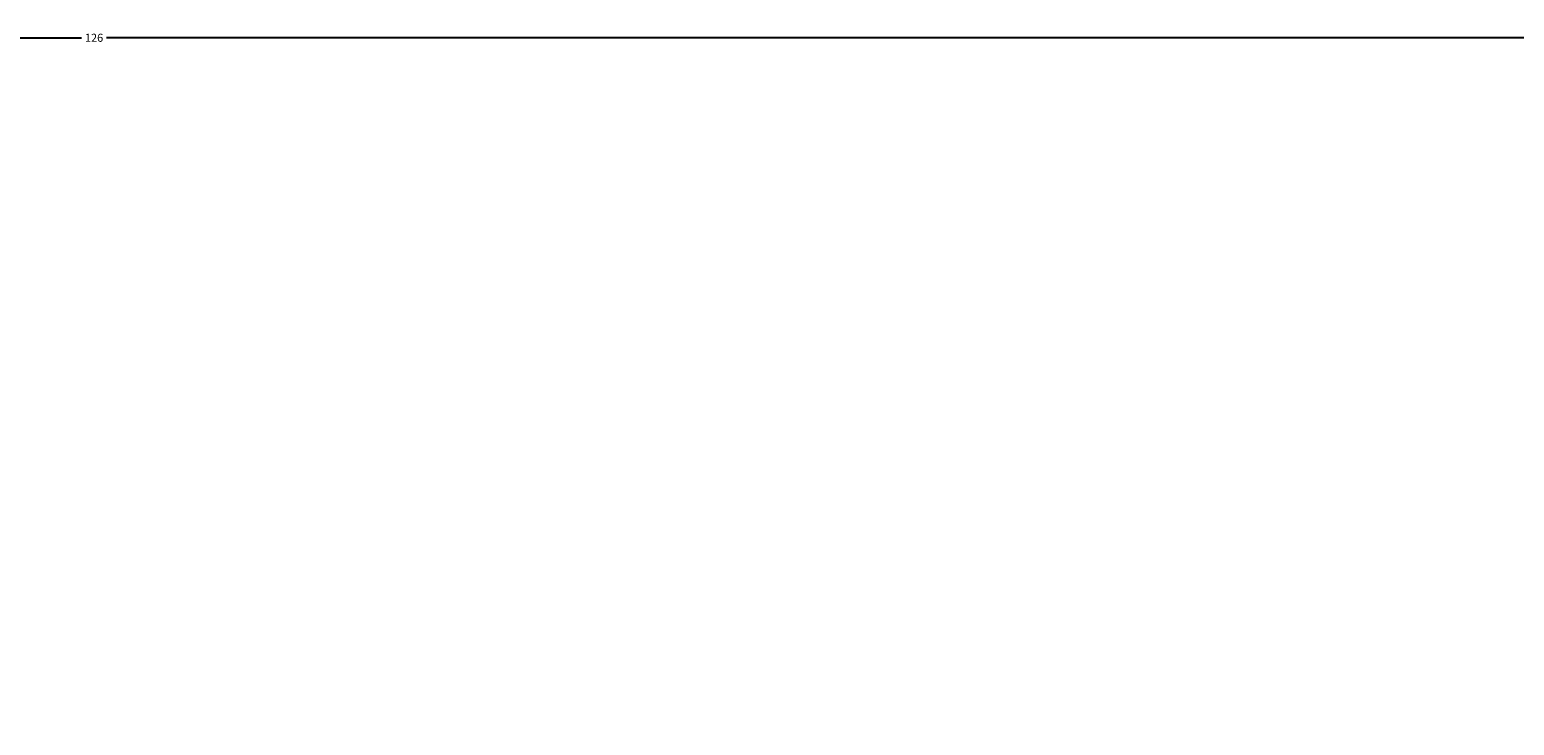
# Model space of a CAD drawing. Units: millimetres. Extents: x -9 to 135, y -119 to 27.
# Tile 9 of 12: x 62 to 95, y 11 to 27. Entities that reach past the tile are written whole.
import ezdxf

# ---------------------------------------------------------------- set-up
doc = ezdxf.new("R2010")
doc.units = ezdxf.units.MM
doc.layers.add('M-DIMS', color=2, linetype='Continuous', lineweight=18)
doc.styles.get("Standard").update_dxf_attribs({"font": 'arial.ttf'})
doc.dimstyles.get("Standard").update_dxf_attribs({"dimtxt": 0.18, "dimasz": 0.18, "dimexe": 0.18, "dimexo": 0.0625, "dimgap": 0.09, "dimtad": 0, "dimtih": 1, "dimtoh": 1, "dimdec": 4, "dimzin": 0, "dimdsep": 46, "dimtxsty": 'Standard', "dimcen": 0.09, "dimadec": 0, "dimazin": 0, "dimtfac": 1, "dimtdec": 4, "dimtofl": 0, "dimtmove": 0, "dimatfit": 3, "dimfxl": 1, "dimtolj": 1, "dimtzin": 0, "dimarcsym": 0})

# ---------------------------------------------------------------- blocks, each defined once
blk = doc.blocks.new('*D2')
at = {"layer": 'Defpoints', "color": 0, "transparency": 16777216}
for p in [(126, 26.533), (0, 17.733), (126, 1.733)]:
    blk.add_point(p, dxfattribs=at)
at = {"layer": 'M-DIMS', "color": 0, "lineweight": -2, "transparency": 16777216}
for p, q in [((0, 17.796), (0, 26.713)), ((126, 1.796), (126, 26.713)), ((0.18, 26.533), (62.72, 26.533)), ((125.82, 26.533), (63.28, 26.533))]:
    blk.add_line(p, q, dxfattribs=at)
at = {"layer": 'M-DIMS', "color": 0, "transparency": 16777216}
for points in [[(0.18, 26.563), (0.18, 26.503), (0, 26.533)], [(125.82, 26.563), (125.82, 26.503), (126, 26.533)]]:
    blk.add_solid(points, dxfattribs=at)
at = {"layer": 'M-DIMS', "color": 0, "transparency": 16777216, "insert": (63, 26.533), "char_height": 0.18, "attachment_point": 5}
blk.add_mtext('\\A1;126', dxfattribs=at)
blk = doc.blocks.new('*D3')
at = {"layer": 'Defpoints', "color": 0, "transparency": 16777216}
for p in [(0, 17.733), (-8.8, -110.267), (63, -110.267)]:
    blk.add_point(p, dxfattribs=at)
at = {"layer": 'M-DIMS', "color": 0, "lineweight": -2, "transparency": 16777216}
for p, q in [((-0.062, 17.733), (-8.98, 17.733)), ((-8.8, 17.553), (-8.8, -46.085)), ((-8.8, -110.087), (-8.8, -46.449)), ((62.938, -110.267), (-8.98, -110.267))]:
    blk.add_line(p, q, dxfattribs=at)
at = {"layer": 'M-DIMS', "color": 0, "transparency": 16777216}
for points in [[(-8.83, 17.553), (-8.77, 17.553), (-8.8, 17.733)], [(-8.83, -110.087), (-8.77, -110.087), (-8.8, -110.267)]]:
    blk.add_solid(points, dxfattribs=at)
at = {"layer": 'M-DIMS', "color": 0, "transparency": 16777216, "insert": (-8.8, -46.267), "char_height": 0.18, "attachment_point": 5}
blk.add_mtext('\\A1;128', dxfattribs=at)

msp = doc.modelspace()

# ---------------------------------------------------------------- dimensions: what is measured, and where the dimension line sits
at = {"layer": 'M-DIMS'}
dim = msp.add_linear_dim(base=(126, 26.533), p1=(0, 17.733), p2=(126, 1.733), dimstyle='Standard', override={"dimdec": 0, "dimlfac": 1, "dimrnd": 0, "dimzin": 0, "dimdsep": 46, "dimlunit": 2}, dxfattribs=at)
dim.commit()
dim.dimension.update_dxf_attribs({"geometry": '*D2', "text_midpoint": (63, 26.533)})
dim = msp.add_linear_dim(base=(-8.8, -110.267), p1=(0, 17.733), p2=(63, -110.267), angle=90, dimstyle='Standard', override={"dimdec": 0, "dimlfac": 1, "dimrnd": 0, "dimzin": 0, "dimdsep": 46, "dimlunit": 2}, dxfattribs=at)
dim.commit()
dim.dimension.update_dxf_attribs({"geometry": '*D3', "text_midpoint": (-8.8, -46.267)})

doc.saveas('drawing.dxf')
